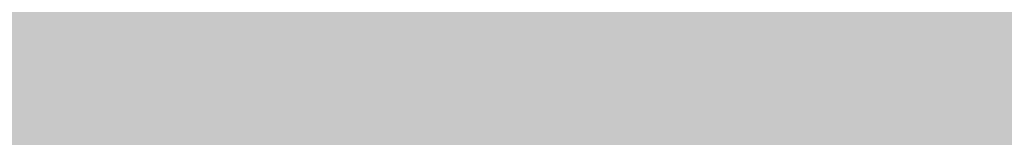
# Model space of a CAD drawing. Units: millimetres. Extents: x 0 to 2267, y 0 to 1823.
# Tile 199 of 256: x 1838.83 to 1841.442, y 1127.462 to 1127.775. Entities that reach past the tile are written whole.
import ezdxf

# ---------------------------------------------------------------- set-up
doc = ezdxf.new("R2010")
doc.units = ezdxf.units.MM
doc.header["$MEASUREMENT"] = 0
doc.layers.add('M-HATC', color=252, linetype='Continuous', lineweight=18)

msp = doc.modelspace()

# ---------------------------------------------------------------- hatches: boundary and pattern name
at = {"layer": 'M-HATC'}
h = msp.add_hatch(color=256, dxfattribs=at)
h.dxf.hatch_style = 1
h.paths.add_polyline_path([(2055.771, 1603.062), (1381.0868, 1603.062), (1381.0868, 1598.062), (2055.771, 1598.062)])
h.paths.add_polyline_path([(2055.771, 1598.062), (1381.0868, 1598.062), (1381.0868, 1593.062), (2055.771, 1593.062)])
h.paths.add_polyline_path([(2051.3074, 1536.7609), (1385.5504, 1536.7609), (1385.5504, 1526.7609), (1387.5504, 1526.7609), (1388.5366, 1525.0528), (1385.3319, 1521.2335), (1385.3319, 1521.2226), (2050.2542, 1522.7491), (2048.3212, 1525.0528), (2049.3074, 1526.7609), (2051.3074, 1526.7609)])
edge = h.paths.add_edge_path()
edge.add_arc((1847.5345, 1379.1492), 135, 222.603061, 222.890851, ccw=False)
edge.add_line((1748.1663, 1287.7656), (1683.0921, 1287.7656))
edge.add_arc((1583.7239, 1379.1492), 135, 317.109149, 317.396939, ccw=False)
edge.add_arc((1678.9686, 1290.6707), 5, 222.8909, 317.1091, ccw=False)
edge.add_arc((1774.2133, 1379.1492), 135, 222.603061, 222.890851, ccw=False)
edge.add_line((1674.8451, 1287.7656), (1609.7709, 1287.7656))
edge.add_arc((1510.4027, 1379.1492), 135, 317.109149, 317.396939, ccw=False)
edge.add_arc((1605.6474, 1290.6707), 5, 222.8909, 317.1091, ccw=False)
edge.add_arc((1700.8921, 1379.1492), 135, 222.603061, 222.890851, ccw=False)
edge.add_line((1601.5239, 1287.7656), (1536.4497, 1287.7656))
edge.add_arc((1437.0815, 1379.1492), 135, 317.109149, 317.396939, ccw=False)
edge.add_arc((1532.3262, 1290.6707), 5, 222.8909, 317.1091, ccw=False)
edge.add_arc((1627.5709, 1379.1492), 135, 222.603061, 222.890851, ccw=False)
edge.add_line((1528.2027, 1287.7656), (1505.9289, 1287.7656))
edge.add_spline(control_points=[(1505.9289, 1287.7656), (1504.2622, 1287.7656), (1504.2622, 1282.7656), (1505.9289, 1282.7656)], knot_values=[0, 0, 0, 0, 5, 5, 5, 5], degree=3, periodic=0)
edge.add_line((1505.9289, 1282.7656), (1930.9289, 1282.7656))
edge.add_spline(control_points=[(1930.9289, 1282.7656), (1932.5956, 1282.7656), (1932.5956, 1287.7656), (1930.9289, 1287.7656)], knot_values=[0, 0, 0, 0, 5, 5, 5, 5], degree=3, periodic=0)
edge.add_line((1930.9289, 1287.7656), (1903.0557, 1287.7656))
edge.add_arc((1803.6875, 1379.1492), 135, 317.109149, 317.396939, ccw=False)
edge.add_arc((1898.9322, 1290.6707), 5, 222.8909, 317.1091, ccw=False)
edge.add_arc((1994.1769, 1379.1492), 135, 222.603061, 222.890851, ccw=False)
edge.add_line((1894.8087, 1287.7656), (1829.7345, 1287.7656))
edge.add_arc((1730.3663, 1379.1492), 135, 317.109149, 317.396939, ccw=False)
edge.add_arc((1825.611, 1290.6707), 5, 222.8909, 317.1091, ccw=False)
edge.add_arc((1920.8557, 1379.1492), 135, 222.603061, 222.890851, ccw=False)
edge.add_line((1821.4875, 1287.7656), (1756.4133, 1287.7656))
edge.add_arc((1657.0451, 1379.1492), 135, 317.109149, 317.396939, ccw=False)
edge.add_arc((1752.2898, 1290.6707), 5, 222.8909, 317.1091, ccw=False)
edge = h.paths.add_edge_path()
edge.add_spline(control_points=[(1843.4289, 1227.2475), (1845.0956, 1227.2475), (1845.0956, 1232.2475), (1843.4289, 1232.2475)], knot_values=[0, 0, 0, 0, 5, 5, 5, 5], degree=3, periodic=0)
edge.add_line((1843.4289, 1232.2475), (1593.4289, 1232.2475))
edge.add_spline(control_points=[(1593.4289, 1232.2475), (1591.7622, 1232.2475), (1591.7622, 1227.2475), (1593.4289, 1227.2475)], knot_values=[0, 0, 0, 0, 5, 5, 5, 5], degree=3, periodic=0)
edge.add_line((1593.4289, 1227.2475), (1843.4289, 1227.2475))
h.paths.add_polyline_path([(1905.9289, 1127.4171), (1530.9289, 1127.4171, 0.414214), (1520.9289, 1117.4171), (1530.9289, 1117.4171), (1915.9289, 1117.4171, 0.414214)])
edge = h.paths.add_edge_path()
edge.add_arc((1397.0858, 1498.4078), 12.7299, 90.78215, 190.87871, ccw=False)
edge.add_line((1396.912, 1511.1365), (1428.0097, 1511.3488))
edge.add_line((1428.0097, 1511.3488), (1433.0097, 1511.3488))
edge.add_line((1433.0097, 1511.3488), (1434.439, 1511.3488))
edge.add_arc((1419.474, 1498.0804), 20, 41.561, 74.08211)
edge.add_line((1424.9592, 1517.3135), (1399.9351, 1517.2561))
edge.add_spline(control_points=[(1399.9307, 1517.2561), (1399.884, 1517.2131), (1399.8328, 1517.1689), (1399.7774, 1517.1236)], knot_values=[11.567499, 11.567499, 11.567499, 11.567499, 11.814249, 11.814249, 11.814249, 11.814249], degree=3, periodic=0)
edge.add_spline(control_points=[(1399.6328, 1517.0099), (1399.5831, 1516.9721), (1399.5307, 1516.9338), (1399.4759, 1516.8947)], knot_values=[11.167718, 11.167718, 11.167718, 11.167718, 11.365188, 11.365188, 11.365188, 11.365188], degree=3, periodic=0)
edge.add_spline(control_points=[(1399.3398, 1516.8001), (1399.1514, 1516.6719), (1398.9384, 1516.5377), (1398.704, 1516.3994)], knot_values=[10.376405, 10.376405, 10.376405, 10.376405, 11.00994, 11.00994, 11.00994, 11.00994], degree=3, periodic=0)
edge.add_spline(control_points=[(1398.6572, 1516.3719), (1398.5789, 1516.326), (1398.4983, 1516.2797), (1398.4155, 1516.2331)], knot_values=[10.125175, 10.125175, 10.125175, 10.125175, 10.334406, 10.334406, 10.334406, 10.334406], degree=3, periodic=0)
edge.add_spline(control_points=[(1398.2642, 1516.1487), (1398.196, 1516.1111), (1398.1263, 1516.0732), (1398.0555, 1516.0351)], knot_values=[9.832246, 9.832246, 9.832246, 9.832246, 9.999658, 9.999658, 9.999658, 9.999658], degree=3, periodic=0)
edge.add_spline(control_points=[(1397.9987, 1516.0048), (1397.7312, 1515.8621), (1397.446, 1515.7171), (1397.1466, 1515.5714)], knot_values=[9.161808, 9.161808, 9.161808, 9.161808, 9.787769, 9.787769, 9.787769, 9.787769], degree=3, periodic=0)
edge.add_spline(control_points=[(1397.1466, 1515.5714), (1396.8418, 1515.423), (1396.5222, 1515.274), (1396.1914, 1515.1262)], knot_values=[8.524455, 8.524455, 8.524455, 8.524455, 9.161808, 9.161808, 9.161808, 9.161808], degree=3, periodic=0)
edge.add_spline(control_points=[(1396.0777, 1515.0756), (1395.9854, 1515.0348), (1395.8922, 1514.994), (1395.7983, 1514.9534)], knot_values=[8.275193, 8.275193, 8.275193, 8.275193, 8.451726, 8.451726, 8.451726, 8.451726], degree=3, periodic=0)
edge.add_spline(control_points=[(1395.6018, 1514.8691), (1395.4997, 1514.8257), (1395.3968, 1514.7824), (1395.2932, 1514.7394)], knot_values=[7.962917, 7.962917, 7.962917, 7.962917, 8.152764, 8.152764, 8.152764, 8.152764], degree=3, periodic=0)
edge.add_spline(control_points=[(1395.2116, 1514.7057), (1394.8278, 1514.5475), (1394.4345, 1514.3929), (1394.0364, 1514.2442)], knot_values=[7.21254, 7.21254, 7.21254, 7.21254, 7.913148, 7.913148, 7.913148, 7.913148], degree=3, periodic=0)
edge.add_spline(control_points=[(1394.0364, 1514.2442), (1393.7076, 1514.1214), (1393.3754, 1514.0027), (1393.0427, 1513.8895)], knot_values=[6.633733, 6.633733, 6.633733, 6.633733, 7.21254, 7.21254, 7.21254, 7.21254], degree=3, periodic=0)
edge.add_spline(control_points=[(1392.8214, 1513.815), (1392.7198, 1513.7812), (1392.6181, 1513.7479), (1392.5166, 1513.7152)], knot_values=[6.328796, 6.328796, 6.328796, 6.328796, 6.505493, 6.505493, 6.505493, 6.505493], degree=3, periodic=0)
edge.add_spline(control_points=[(1392.5166, 1513.7152), (1392.3187, 1513.6515), (1392.1212, 1513.59), (1391.9244, 1513.531)], knot_values=[5.984605, 5.984605, 5.984605, 5.984605, 6.328796, 6.328796, 6.328796, 6.328796], degree=3, periodic=0)
edge.add_spline(control_points=[(1391.7915, 1513.4915), (1391.3122, 1513.3501), (1390.8384, 1513.2239), (1390.3784, 1513.1171)], knot_values=[5.066697, 5.066697, 5.066697, 5.066697, 5.907055, 5.907055, 5.907055, 5.907055], degree=3, periodic=0)
edge.add_spline(control_points=[(1390.3784, 1513.1171), (1390.1797, 1513.071), (1389.9836, 1513.0284), (1389.7907, 1512.9899)], knot_values=[4.70367, 4.70367, 4.70367, 4.70367, 5.066695, 5.066695, 5.066695, 5.066695], degree=3, periodic=0)
edge.add_spline(control_points=[(1389.422, 1512.9204), (1389.2459, 1512.8892), (1389.0729, 1512.8617), (1388.9036, 1512.8381)], knot_values=[4.130571, 4.130571, 4.130571, 4.130571, 4.469816, 4.469816, 4.469816, 4.469816], degree=3, periodic=0)
edge.add_spline(control_points=[(1388.9036, 1512.8381), (1388.591, 1512.7946), (1388.2911, 1512.7644), (1388.0071, 1512.7494)], knot_values=[3.504031, 3.504031, 3.504031, 3.504031, 4.130571, 4.130571, 4.130571, 4.130571], degree=3, periodic=0)
edge.add_spline(control_points=[(1387.9356, 1512.7459), (1387.8538, 1512.7423), (1387.7733, 1512.74), (1387.6944, 1512.739)], knot_values=[3.268866, 3.268866, 3.268866, 3.268866, 3.451164, 3.451164, 3.451164, 3.451164], degree=3, periodic=0)
edge.add_spline(control_points=[(1387.3351, 1512.7443), (1387.2076, 1512.7499), (1387.0847, 1512.7597), (1386.967, 1512.7739)], knot_values=[2.670686, 2.670686, 2.670686, 2.670686, 2.984, 2.984, 2.984, 2.984], degree=3, periodic=0)
edge.add_spline(control_points=[(1386.8327, 1512.7922), (1386.8209, 1512.7941), (1386.8092, 1512.7959), (1386.7975, 1512.7979)], knot_values=[2.516981, 2.516981, 2.516981, 2.516981, 2.549528, 2.549528, 2.549528, 2.549528], degree=3, periodic=0)
edge.add_spline(control_points=[(1386.4526, 1512.8735), (1386.4257, 1512.881), (1386.3993, 1512.889), (1386.3733, 1512.8972)], knot_values=[2.095869, 2.095869, 2.095869, 2.095869, 2.17941, 2.17941, 2.17941, 2.17941], degree=3, periodic=0)
edge.add_spline(control_points=[(1386.0691, 1513.0189), (1386.0634, 1513.0217), (1386.0577, 1513.0246), (1386.052, 1513.0275)], knot_values=[1.72453, 1.72453, 1.72453, 1.72453, 1.745933, 1.745933, 1.745933, 1.745933], degree=3, periodic=0)
edge.add_arc((1399.474, 1498.0804), 20, 131.82432, 180)
edge.add_arc((1630.3336, 1505.5484), 250.9708, 181.705176, 236.427975)
edge.add_arc((1605.3399, 1483.3044), 218.7822, 238.660829, 243.34961)
edge.add_arc((1647.0911, 1510.3592), 262.8986, 183.129836, 237.853442, ccw=False)
h.paths.add_polyline_path([(1406.5369, 1391.9644, 0.149382), (1491.5506, 1296.4418, -0.129517)], flags=17)
edge = h.paths.add_edge_path()
edge.add_arc((2037.3838, 1498.0804), 20, 0, 48.26587)
edge.add_spline(control_points=[(2050.6973, 1513.0052), (2050.6512, 1512.9847), (2050.6034, 1512.9655), (2050.5539, 1512.9477)], knot_values=[1.835652, 1.835652, 1.835652, 1.835652, 2.000781, 2.000781, 2.000781, 2.000781], degree=3, periodic=0)
edge.add_spline(control_points=[(2050.4616, 1512.9166), (2050.479, 1512.9221), (2050.4963, 1512.9277), (2050.5133, 1512.9335)], knot_values=[2.045477, 2.045477, 2.045477, 2.045477, 2.101389, 2.101389, 2.101389, 2.101389], degree=3, periodic=0)
edge.add_spline(control_points=[(2050.129, 1512.8342), (2050.1984, 1512.8473), (2050.2657, 1512.8623), (2050.3308, 1512.8792)], knot_values=[2.237629, 2.237629, 2.237629, 2.237629, 2.435841, 2.435841, 2.435841, 2.435841], degree=3, periodic=0)
edge.add_spline(control_points=[(2050.0946, 1512.8278), (2050.1061, 1512.8299), (2050.1176, 1512.832), (2050.129, 1512.8342)], knot_values=[2.435841, 2.435841, 2.435841, 2.435841, 2.468321, 2.468321, 2.468321, 2.468321], degree=3, periodic=0)
edge.add_spline(control_points=[(2049.7843, 1512.7851), (2049.8552, 1512.7922), (2049.9243, 1512.8008), (2049.9917, 1512.8109)], knot_values=[2.563852, 2.563852, 2.563852, 2.563852, 2.748541, 2.748541, 2.748541, 2.748541], degree=3, periodic=0)
edge.add_spline(control_points=[(2049.4052, 1512.7617), (2049.5364, 1512.7653), (2049.6629, 1512.773), (2049.7843, 1512.7851)], knot_values=[2.748541, 2.748541, 2.748541, 2.748541, 3.064882, 3.064882, 3.064882, 3.064882], degree=3, periodic=0)
edge.add_spline(control_points=[(2049.1698, 1512.7597), (2049.2336, 1512.7591), (2049.2965, 1512.7594), (2049.3584, 1512.7606)], knot_values=[3.102309, 3.102309, 3.102309, 3.102309, 3.2503, 3.2503, 3.2503, 3.2503], degree=3, periodic=0)
edge.add_spline(control_points=[(2048.8573, 1512.7691), (2048.9638, 1512.7638), (2049.068, 1512.7606), (2049.1698, 1512.7597)], knot_values=[3.2503, 3.2503, 3.2503, 3.2503, 3.486069, 3.486069, 3.486069, 3.486069], degree=3, periodic=0)
edge.add_spline(control_points=[(2048.6924, 1512.7789), (2048.3729, 1512.8009), (2048.0345, 1512.8411), (2047.6817, 1512.897)], knot_values=[3.606429, 3.606429, 3.606429, 3.606429, 4.2989, 4.2989, 4.2989, 4.2989], degree=3, periodic=0)
edge.add_spline(control_points=[(2047.6817, 1512.897), (2047.5458, 1512.9185), (2047.4077, 1512.9424), (2047.2678, 1512.9685)], knot_values=[4.2989, 4.2989, 4.2989, 4.2989, 4.565769, 4.565769, 4.565769, 4.565769], degree=3, periodic=0)
edge.add_spline(control_points=[(2047.2678, 1512.9685), (2047.1449, 1512.9914), (2047.0207, 1513.016), (2046.8951, 1513.0422)], knot_values=[4.565769, 4.565769, 4.565769, 4.565769, 4.799971, 4.799971, 4.799971, 4.799971], degree=3, periodic=0)
edge.add_spline(control_points=[(2046.8951, 1513.0422), (2046.5286, 1513.1188), (2046.1513, 1513.209), (2045.7676, 1513.3107)], knot_values=[4.799971, 4.799971, 4.799971, 4.799971, 5.483718, 5.483718, 5.483718, 5.483718], degree=3, periodic=0)
edge.add_spline(control_points=[(2045.7676, 1513.3107), (2045.3724, 1513.4154), (2044.9704, 1513.5322), (2044.5662, 1513.6588)], knot_values=[5.483718, 5.483718, 5.483718, 5.483718, 6.187866, 6.187866, 6.187866, 6.187866], degree=3, periodic=0)
edge.add_spline(control_points=[(2044.5662, 1513.6588), (2044.4149, 1513.7061), (2044.2633, 1513.7549), (2044.1116, 1513.8048)], knot_values=[6.187866, 6.187866, 6.187866, 6.187866, 6.451551, 6.451551, 6.451551, 6.451551], degree=3, periodic=0)
edge.add_spline(control_points=[(2044.1116, 1513.8048), (2043.9967, 1513.8427), (2043.8817, 1513.8813), (2043.7668, 1513.9205)], knot_values=[6.451551, 6.451551, 6.451551, 6.451551, 6.651434, 6.651434, 6.651434, 6.651434], degree=3, periodic=0)
edge.add_spline(control_points=[(2043.7668, 1513.9205), (2043.3716, 1514.0554), (2042.9774, 1514.1979), (2042.5886, 1514.3458)], knot_values=[6.651434, 6.651434, 6.651434, 6.651434, 7.338879, 7.338879, 7.338879, 7.338879], degree=3, periodic=0)
edge.add_spline(control_points=[(2042.5886, 1514.3458), (2042.1643, 1514.5071), (2041.7465, 1514.6749), (2041.3409, 1514.846)], knot_values=[7.338879, 7.338879, 7.338879, 7.338879, 8.089209, 8.089209, 8.089209, 8.089209], degree=3, periodic=0)
edge.add_spline(control_points=[(2041.3409, 1514.846), (2041.1028, 1514.9465), (2040.869, 1515.0481), (2040.6405, 1515.1502)], knot_values=[8.089209, 8.089209, 8.089209, 8.089209, 8.529587, 8.529587, 8.529587, 8.529587], degree=3, periodic=0)
edge.add_spline(control_points=[(2040.51, 1515.2089), (2040.0824, 1515.4022), (2039.6747, 1515.5971), (2039.295, 1515.7894)], knot_values=[8.613818, 8.613818, 8.613818, 8.613818, 9.44571, 9.44571, 9.44571, 9.44571], degree=3, periodic=0)
edge.add_spline(control_points=[(2039.295, 1515.7894), (2039.0618, 1515.9075), (2038.8391, 1516.0246), (2038.6288, 1516.1398)], knot_values=[9.44571, 9.44571, 9.44571, 9.44571, 9.956404, 9.956404, 9.956404, 9.956404], degree=3, periodic=0)
edge.add_spline(control_points=[(2038.6288, 1516.1398), (2038.5187, 1516.2001), (2038.4121, 1516.2598), (2038.309, 1516.3189)], knot_values=[9.956404, 9.956404, 9.956404, 9.956404, 10.223542, 10.223542, 10.223542, 10.223542], degree=3, periodic=0)
edge.add_spline(control_points=[(2038.309, 1516.3189), (2038.2138, 1516.3735), (2038.1216, 1516.4276), (2038.0328, 1516.481)], knot_values=[10.223542, 10.223542, 10.223542, 10.223542, 10.47051, 10.47051, 10.47051, 10.47051], degree=3, periodic=0)
edge.add_spline(control_points=[(2038.0328, 1516.481), (2037.7855, 1516.6296), (2037.5639, 1516.773), (2037.3722, 1516.909)], knot_values=[10.47051, 10.47051, 10.47051, 10.47051, 11.15767, 11.15767, 11.15767, 11.15767], degree=3, periodic=0)
edge.add_spline(control_points=[(2037.3722, 1516.909), (2037.2789, 1516.9752), (2037.1927, 1517.0396), (2037.1142, 1517.102)], knot_values=[11.15767, 11.15767, 11.15767, 11.15767, 11.49227, 11.49227, 11.49227, 11.49227], degree=3, periodic=0)
edge.add_spline(control_points=[(2036.8564, 1517.3259), (2036.9148, 1517.2692), (2036.9814, 1517.2103), (2037.0557, 1517.1492)], knot_values=[11.577341, 11.577341, 11.577341, 11.577341, 11.91035, 11.91035, 11.91035, 11.91035], degree=3, periodic=0)
edge.add_spline(control_points=[(2036.8074, 1517.3748), (2036.823, 1517.3587), (2036.8393, 1517.3424), (2036.8564, 1517.3259)], knot_values=[11.91035, 11.91035, 11.91035, 11.91035, 12.007402, 12.007402, 12.007402, 12.007402], degree=3, periodic=0)
edge.add_spline(control_points=[(2036.7017, 1517.494), (2036.7104, 1517.483), (2036.7196, 1517.4719), (2036.7291, 1517.4606)], knot_values=[12.184155, 12.184155, 12.184155, 12.184155, 12.255409, 12.255409, 12.255409, 12.255409], degree=3, periodic=0)
edge.add_spline(control_points=[(2036.6159, 1517.6205), (2036.62, 1517.613), (2036.6243, 1517.6055), (2036.6289, 1517.5979)], knot_values=[12.487913, 12.487913, 12.487913, 12.487913, 12.541035, 12.541035, 12.541035, 12.541035], degree=3, periodic=0)
edge.add_spline(control_points=[(2036.5635, 1517.786), (2036.5637, 1517.7794), (2036.5642, 1517.7726), (2036.565, 1517.7658)], knot_values=[12.911761, 12.911761, 12.911761, 12.911761, 12.968286, 12.968286, 12.968286, 12.968286], degree=3, periodic=0)
edge.add_spline(control_points=[(2036.6166, 1517.9304), (2036.6125, 1517.9259), (2036.6086, 1517.9212), (2036.6049, 1517.9165)], knot_values=[13.382527, 13.382527, 13.382527, 13.382527, 13.433791, 13.433791, 13.433791, 13.433791], degree=3, periodic=0)
edge.add_spline(control_points=[(2036.749, 1518.017), (2036.7361, 1518.0116), (2036.7239, 1518.006), (2036.7124, 1518.0002)], knot_values=[13.726299, 13.726299, 13.726299, 13.726299, 13.809928, 13.809928, 13.809928, 13.809928], degree=3, periodic=0)
edge.add_spline(control_points=[(2036.8604, 1518.0528), (2036.8386, 1518.0474), (2036.8181, 1518.0416), (2036.7988, 1518.0353)], knot_values=[13.910887, 13.910887, 13.910887, 13.910887, 14.02153, 14.02153, 14.02153, 14.02153], degree=3, periodic=0)
edge.add_line((2036.9639, 1518.0804), (2032.3838, 1518.0804))
edge.add_line((2032.3838, 1518.0804), (2027.3838, 1518.0804))
edge.add_line((2027.3838, 1518.0804), (2022.3838, 1518.0804))
edge.add_line((2022.3838, 1518.0804), (2017.3838, 1518.0804))
edge.add_arc((2017.3838, 1498.0804), 20, 90, 138.439)
edge.add_line((2002.4188, 1511.3488), (2003.8481, 1511.3488))
edge.add_line((2003.8481, 1511.3488), (2008.8481, 1511.3488))
edge.add_line((2008.8481, 1511.3488), (2039.772, 1511.1377))
edge.add_arc((2039.772, 1498.4078), 12.7299, -10.87871, 90, ccw=False)
edge.add_arc((1789.7668, 1510.3592), 262.8986, 302.146558, 356.870164, ccw=False)
edge.add_arc((1831.5179, 1483.3044), 218.7822, 296.65039, 301.339171)
edge.add_arc((1806.5242, 1505.5484), 250.9708, 303.572025, 358.294824)
h.paths.add_polyline_path([(2030.321, 1391.9644, -0.129517), (1945.3072, 1296.4418, 0.149382)], flags=17)
edge = h.paths.add_edge_path()
edge.add_spline(control_points=[(2037.2464, 1518.0821), (2037.2898, 1518.081), (2037.3355, 1518.0804), (2037.3838, 1518.0804)], knot_values=[0.000012, 0.000012, 0.000012, 0.000012, 0.144754, 0.144754, 0.144754, 0.144754], degree=3, periodic=0)
edge.add_line((2037.3357, 1518.0804), (2037.0096, 1518.0804))
edge.add_spline(control_points=[(2037.0096, 1518.0804), (2036.9822, 1518.0768), (2036.956, 1518.0727), (2036.9312, 1518.0681)], knot_values=[14.13465, 14.13465, 14.13465, 14.13465, 14.247197, 14.247197, 14.247197, 14.247197], degree=3, periodic=0)
edge.add_spline(control_points=[(2036.9312, 1518.0681), (2036.9276, 1518.0674), (2036.9241, 1518.0667), (2036.9205, 1518.0661)], knot_values=[14.118315, 14.118315, 14.118315, 14.118315, 14.13465, 14.13465, 14.13465, 14.13465], degree=3, periodic=0)
edge.add_spline(control_points=[(2036.9205, 1518.0661), (2036.9118, 1518.0644), (2036.9032, 1518.0626), (2036.8948, 1518.0608)], knot_values=[14.078086, 14.078086, 14.078086, 14.078086, 14.118315, 14.118315, 14.118315, 14.118315], degree=3, periodic=0)
edge.add_spline(control_points=[(2036.8948, 1518.0608), (2036.883, 1518.0583), (2036.8716, 1518.0556), (2036.8604, 1518.0528)], knot_values=[14.02153, 14.02153, 14.02153, 14.02153, 14.078086, 14.078086, 14.078086, 14.078086], degree=3, periodic=0)
edge.add_spline(control_points=[(2036.8604, 1518.0528), (2036.8386, 1518.0474), (2036.8181, 1518.0416), (2036.7988, 1518.0353)], knot_values=[13.910887, 13.910887, 13.910887, 13.910887, 14.02153, 14.02153, 14.02153, 14.02153], degree=3, periodic=0)
edge.add_spline(control_points=[(2036.7988, 1518.0353), (2036.7981, 1518.035), (2036.7974, 1518.0348), (2036.7967, 1518.0346)], knot_values=[13.906906, 13.906906, 13.906906, 13.906906, 13.910887, 13.910887, 13.910887, 13.910887], degree=3, periodic=0)
edge.add_spline(control_points=[(2036.7967, 1518.0346), (2036.7882, 1518.0318), (2036.7799, 1518.0289), (2036.7719, 1518.0259)], knot_values=[13.857826, 13.857826, 13.857826, 13.857826, 13.906906, 13.906906, 13.906906, 13.906906], degree=3, periodic=0)
edge.add_spline(control_points=[(2036.7719, 1518.0259), (2036.764, 1518.023), (2036.7564, 1518.02), (2036.749, 1518.017)], knot_values=[13.809928, 13.809928, 13.809928, 13.809928, 13.857826, 13.857826, 13.857826, 13.857826], degree=3, periodic=0)
edge.add_spline(control_points=[(2036.749, 1518.017), (2036.7361, 1518.0116), (2036.7239, 1518.006), (2036.7124, 1518.0002)], knot_values=[13.726299, 13.726299, 13.726299, 13.726299, 13.809928, 13.809928, 13.809928, 13.809928], degree=3, periodic=0)
edge.add_spline(control_points=[(2036.7124, 1518.0002), (2036.7121, 1518), (2036.7118, 1517.9999), (2036.7115, 1517.9997)], knot_values=[13.723993, 13.723993, 13.723993, 13.723993, 13.726299, 13.726299, 13.726299, 13.726299], degree=3, periodic=0)
edge.add_spline(control_points=[(2036.7115, 1517.9997), (2036.7063, 1517.9971), (2036.7013, 1517.9944), (2036.6965, 1517.9917)], knot_values=[13.686536, 13.686536, 13.686536, 13.686536, 13.723993, 13.723993, 13.723993, 13.723993], degree=3, periodic=0)
edge.add_spline(control_points=[(2036.6965, 1517.9917), (2036.6919, 1517.9891), (2036.6874, 1517.9865), (2036.6831, 1517.9839)], knot_values=[13.651251, 13.651251, 13.651251, 13.651251, 13.686536, 13.686536, 13.686536, 13.686536], degree=3, periodic=0)
edge.add_spline(control_points=[(2036.6831, 1517.9839), (2036.6764, 1517.9798), (2036.67, 1517.9757), (2036.6639, 1517.9714)], knot_values=[13.596804, 13.596804, 13.596804, 13.596804, 13.651251, 13.651251, 13.651251, 13.651251], degree=3, periodic=0)
edge.add_spline(control_points=[(2036.6639, 1517.9714), (2036.6636, 1517.9712), (2036.6633, 1517.9709), (2036.6629, 1517.9707)], knot_values=[13.593956, 13.593956, 13.593956, 13.593956, 13.596804, 13.596804, 13.596804, 13.596804], degree=3, periodic=0)
edge.add_spline(control_points=[(2036.6629, 1517.9707), (2036.6603, 1517.9689), (2036.6577, 1517.967), (2036.6552, 1517.9651)], knot_values=[13.570322, 13.570322, 13.570322, 13.570322, 13.593956, 13.593956, 13.593956, 13.593956], degree=3, periodic=0)
edge.add_spline(control_points=[(2036.6552, 1517.9651), (2036.6525, 1517.9631), (2036.6499, 1517.9611), (2036.6474, 1517.9591)], knot_values=[13.545477, 13.545477, 13.545477, 13.545477, 13.570322, 13.570322, 13.570322, 13.570322], degree=3, periodic=0)
edge.add_spline(control_points=[(2036.6474, 1517.9591), (2036.6472, 1517.9589), (2036.6471, 1517.9588), (2036.6469, 1517.9587)], knot_values=[13.543931, 13.543931, 13.543931, 13.543931, 13.545477, 13.545477, 13.545477, 13.545477], degree=3, periodic=0)
edge.add_spline(control_points=[(2036.6469, 1517.9587), (2036.6412, 1517.9541), (2036.6358, 1517.9494), (2036.6307, 1517.9447)], knot_values=[13.488237, 13.488237, 13.488237, 13.488237, 13.543931, 13.543931, 13.543931, 13.543931], degree=3, periodic=0)
edge.add_spline(control_points=[(2036.6307, 1517.9447), (2036.6282, 1517.9423), (2036.6257, 1517.9399), (2036.6233, 1517.9374)], knot_values=[13.460307, 13.460307, 13.460307, 13.460307, 13.488237, 13.488237, 13.488237, 13.488237], degree=3, periodic=0)
edge.add_spline(control_points=[(2036.6233, 1517.9374), (2036.6215, 1517.9356), (2036.6198, 1517.9338), (2036.6181, 1517.932)], knot_values=[13.439712, 13.439712, 13.439712, 13.439712, 13.460307, 13.460307, 13.460307, 13.460307], degree=3, periodic=0)
edge.add_spline(control_points=[(2036.6181, 1517.932), (2036.6176, 1517.9315), (2036.6171, 1517.9309), (2036.6166, 1517.9304)], knot_values=[13.433791, 13.433791, 13.433791, 13.433791, 13.439712, 13.439712, 13.439712, 13.439712], degree=3, periodic=0)
edge.add_spline(control_points=[(2036.6166, 1517.9304), (2036.6125, 1517.9259), (2036.6086, 1517.9212), (2036.6049, 1517.9165)], knot_values=[13.382527, 13.382527, 13.382527, 13.382527, 13.433791, 13.433791, 13.433791, 13.433791], degree=3, periodic=0)
edge.add_spline(control_points=[(2036.6049, 1517.9165), (2036.6026, 1517.9135), (2036.6004, 1517.9104), (2036.5982, 1517.9074)], knot_values=[13.350017, 13.350017, 13.350017, 13.350017, 13.382527, 13.382527, 13.382527, 13.382527], degree=3, periodic=0)
edge.add_spline(control_points=[(2036.5982, 1517.9074), (2036.5972, 1517.9059), (2036.5962, 1517.9043), (2036.5952, 1517.9028)], knot_values=[13.333922, 13.333922, 13.333922, 13.333922, 13.350017, 13.350017, 13.350017, 13.350017], degree=3, periodic=0)
edge.add_spline(control_points=[(2036.5952, 1517.9028), (2036.5945, 1517.9018), (2036.5939, 1517.9009), (2036.5933, 1517.8999)], knot_values=[13.323828, 13.323828, 13.323828, 13.323828, 13.333922, 13.333922, 13.333922, 13.333922], degree=3, periodic=0)
edge.add_spline(control_points=[(2036.5933, 1517.8999), (2036.5905, 1517.8955), (2036.5879, 1517.8909), (2036.5855, 1517.8864)], knot_values=[13.277545, 13.277545, 13.277545, 13.277545, 13.323828, 13.323828, 13.323828, 13.323828], degree=3, periodic=0)
edge.add_spline(control_points=[(2036.5855, 1517.8864), (2036.5836, 1517.8827), (2036.5817, 1517.8789), (2036.5801, 1517.8751)], knot_values=[13.240119, 13.240119, 13.240119, 13.240119, 13.277545, 13.277545, 13.277545, 13.277545], degree=3, periodic=0)
edge.add_spline(control_points=[(2036.5801, 1517.8751), (2036.5795, 1517.8739), (2036.579, 1517.8727), (2036.5785, 1517.8715)], knot_values=[13.228211, 13.228211, 13.228211, 13.228211, 13.240119, 13.240119, 13.240119, 13.240119], degree=3, periodic=0)
edge.add_spline(control_points=[(2036.5785, 1517.8715), (2036.578, 1517.8702), (2036.5774, 1517.869), (2036.5769, 1517.8677)], knot_values=[13.215717, 13.215717, 13.215717, 13.215717, 13.228211, 13.228211, 13.228211, 13.228211], degree=3, periodic=0)
edge.add_spline(control_points=[(2036.5769, 1517.8677), (2036.5755, 1517.864), (2036.5741, 1517.8603), (2036.5729, 1517.8565)], knot_values=[13.179847, 13.179847, 13.179847, 13.179847, 13.215717, 13.215717, 13.215717, 13.215717], degree=3, periodic=0)
edge.add_spline(control_points=[(2036.5729, 1517.8565), (2036.5713, 1517.8515), (2036.5699, 1517.8464), (2036.5687, 1517.8413)], knot_values=[13.132017, 13.132017, 13.132017, 13.132017, 13.179847, 13.179847, 13.179847, 13.179847], degree=3, periodic=0)
edge.add_spline(control_points=[(2036.5687, 1517.8413), (2036.5684, 1517.8402), (2036.5682, 1517.8392), (2036.568, 1517.8382)], knot_values=[13.122482, 13.122482, 13.122482, 13.122482, 13.132017, 13.132017, 13.132017, 13.132017], degree=3, periodic=0)
edge.add_spline(control_points=[(2036.568, 1517.8382), (2036.5676, 1517.8363), (2036.5672, 1517.8345), (2036.5669, 1517.8327)], knot_values=[13.105592, 13.105592, 13.105592, 13.105592, 13.122482, 13.122482, 13.122482, 13.122482], degree=3, periodic=0)
edge.add_spline(control_points=[(2036.5669, 1517.8327), (2036.5662, 1517.8292), (2036.5657, 1517.8257), (2036.5652, 1517.8222)], knot_values=[13.074063, 13.074063, 13.074063, 13.074063, 13.105592, 13.105592, 13.105592, 13.105592], degree=3, periodic=0)
edge.add_spline(control_points=[(2036.5652, 1517.8222), (2036.5652, 1517.8222), (2036.5652, 1517.8222), (2036.5652, 1517.8222)], knot_values=[13.074043, 13.074043, 13.074043, 13.074043, 13.074063, 13.074063, 13.074063, 13.074063], degree=3, periodic=0)
edge.add_spline(control_points=[(2036.5652, 1517.8222), (2036.5644, 1517.8164), (2036.5639, 1517.8106), (2036.5636, 1517.8046)], knot_values=[13.021884, 13.021884, 13.021884, 13.021884, 13.074043, 13.074043, 13.074043, 13.074043], degree=3, periodic=0)
edge.add_spline(control_points=[(2036.5636, 1517.8046), (2036.5636, 1517.804), (2036.5636, 1517.8034), (2036.5635, 1517.8028)], knot_values=[13.01674, 13.01674, 13.01674, 13.01674, 13.021884, 13.021884, 13.021884, 13.021884], degree=3, periodic=0)
edge.add_spline(control_points=[(2036.5635, 1517.8028), (2036.5634, 1517.8005), (2036.5634, 1517.7982), (2036.5634, 1517.7958)], knot_values=[12.996438, 12.996438, 12.996438, 12.996438, 13.01674, 13.01674, 13.01674, 13.01674], degree=3, periodic=0)
edge.add_spline(control_points=[(2036.5634, 1517.7958), (2036.5633, 1517.7926), (2036.5634, 1517.7893), (2036.5635, 1517.786)], knot_values=[12.968286, 12.968286, 12.968286, 12.968286, 12.996438, 12.996438, 12.996438, 12.996438], degree=3, periodic=0)
edge.add_spline(control_points=[(2036.5635, 1517.786), (2036.5637, 1517.7794), (2036.5642, 1517.7726), (2036.565, 1517.7658)], knot_values=[12.911761, 12.911761, 12.911761, 12.911761, 12.968286, 12.968286, 12.968286, 12.968286], degree=3, periodic=0)
edge.add_spline(control_points=[(2036.565, 1517.7658), (2036.565, 1517.7657), (2036.565, 1517.7656), (2036.565, 1517.7656)], knot_values=[12.911017, 12.911017, 12.911017, 12.911017, 12.911761, 12.911761, 12.911761, 12.911761], degree=3, periodic=0)
edge.add_spline(control_points=[(2036.565, 1517.7656), (2036.5654, 1517.7625), (2036.5658, 1517.7593), (2036.5663, 1517.7562)], knot_values=[12.88528, 12.88528, 12.88528, 12.88528, 12.911017, 12.911017, 12.911017, 12.911017], degree=3, periodic=0)
edge.add_spline(control_points=[(2036.5663, 1517.7562), (2036.5667, 1517.7534), (2036.5672, 1517.7506), (2036.5677, 1517.7478)], knot_values=[12.862519, 12.862519, 12.862519, 12.862519, 12.88528, 12.88528, 12.88528, 12.88528], degree=3, periodic=0)
edge.add_spline(control_points=[(2036.5677, 1517.7478), (2036.5678, 1517.7474), (2036.5679, 1517.7469), (2036.568, 1517.7465)], knot_values=[12.858885, 12.858885, 12.858885, 12.858885, 12.862519, 12.862519, 12.862519, 12.862519], degree=3, periodic=0)
edge.add_spline(control_points=[(2036.568, 1517.7465), (2036.5692, 1517.7399), (2036.5707, 1517.7332), (2036.5724, 1517.7264)], knot_values=[12.8053, 12.8053, 12.8053, 12.8053, 12.858885, 12.858885, 12.858885, 12.858885], degree=3, periodic=0)
edge.add_spline(control_points=[(2036.5724, 1517.7264), (2036.5734, 1517.7226), (2036.5745, 1517.7187), (2036.5756, 1517.7149)], knot_values=[12.775176, 12.775176, 12.775176, 12.775176, 12.8053, 12.8053, 12.8053, 12.8053], degree=3, periodic=0)
edge.add_spline(control_points=[(2036.5756, 1517.7149), (2036.5763, 1517.7125), (2036.577, 1517.7102), (2036.5778, 1517.7078)], knot_values=[12.756759, 12.756759, 12.756759, 12.756759, 12.775176, 12.775176, 12.775176, 12.775176], degree=3, periodic=0)
edge.add_spline(control_points=[(2036.5778, 1517.7078), (2036.5781, 1517.7067), (2036.5784, 1517.7057), (2036.5787, 1517.7047)], knot_values=[12.748742, 12.748742, 12.748742, 12.748742, 12.756759, 12.756759, 12.756759, 12.756759], degree=3, periodic=0)
edge.add_spline(control_points=[(2036.5787, 1517.7047), (2036.5808, 1517.6983), (2036.5831, 1517.6919), (2036.5856, 1517.6854)], knot_values=[12.69959, 12.69959, 12.69959, 12.69959, 12.748742, 12.748742, 12.748742, 12.748742], degree=3, periodic=0)
edge.add_spline(control_points=[(2036.5856, 1517.6854), (2036.5876, 1517.68), (2036.5898, 1517.6746), (2036.5921, 1517.6692)], knot_values=[12.659038, 12.659038, 12.659038, 12.659038, 12.69959, 12.69959, 12.69959, 12.69959], degree=3, periodic=0)
edge.add_spline(control_points=[(2036.5921, 1517.6692), (2036.594, 1517.6648), (2036.5959, 1517.6605), (2036.5979, 1517.6561)], knot_values=[12.626806, 12.626806, 12.626806, 12.626806, 12.659038, 12.659038, 12.659038, 12.659038], degree=3, periodic=0)
edge.add_spline(control_points=[(2036.5979, 1517.6561), (2036.5984, 1517.6551), (2036.5989, 1517.6541), (2036.5993, 1517.6531)], knot_values=[12.619394, 12.619394, 12.619394, 12.619394, 12.626806, 12.626806, 12.626806, 12.626806], degree=3, periodic=0)
edge.add_spline(control_points=[(2036.5993, 1517.6531), (2036.6043, 1517.6424), (2036.6099, 1517.6315), (2036.6159, 1517.6205)], knot_values=[12.541039, 12.541039, 12.541039, 12.541039, 12.619394, 12.619394, 12.619394, 12.619394], degree=3, periodic=0)
edge.add_spline(control_points=[(2036.6159, 1517.6205), (2036.6159, 1517.6205), (2036.6159, 1517.6205), (2036.6159, 1517.6205)], knot_values=[12.541035, 12.541035, 12.541035, 12.541035, 12.541039, 12.541039, 12.541039, 12.541039], degree=3, periodic=0)
edge.add_spline(control_points=[(2036.6159, 1517.6205), (2036.62, 1517.613), (2036.6243, 1517.6055), (2036.6289, 1517.5979)], knot_values=[12.487913, 12.487913, 12.487913, 12.487913, 12.541035, 12.541035, 12.541035, 12.541035], degree=3, periodic=0)
edge.add_spline(control_points=[(2036.6289, 1517.5979), (2036.6326, 1517.5916), (2036.6365, 1517.5853), (2036.6406, 1517.5789)], knot_values=[12.443982, 12.443982, 12.443982, 12.443982, 12.487913, 12.487913, 12.487913, 12.487913], degree=3, periodic=0)
edge.add_spline(control_points=[(2036.6406, 1517.5789), (2036.6414, 1517.5776), (2036.6423, 1517.5763), (2036.6431, 1517.5749)], knot_values=[12.434996, 12.434996, 12.434996, 12.434996, 12.443982, 12.443982, 12.443982, 12.443982], degree=3, periodic=0)
edge.add_spline(control_points=[(2036.6431, 1517.5749), (2036.6531, 1517.5596), (2036.6639, 1517.5439), (2036.6756, 1517.528)], knot_values=[12.329647, 12.329647, 12.329647, 12.329647, 12.434996, 12.434996, 12.434996, 12.434996], degree=3, periodic=0)
edge.add_spline(control_points=[(2036.6756, 1517.528), (2036.6839, 1517.5168), (2036.6925, 1517.5055), (2036.7017, 1517.494)], knot_values=[12.255409, 12.255409, 12.255409, 12.255409, 12.329647, 12.329647, 12.329647, 12.329647], degree=3, periodic=0)
edge.add_spline(control_points=[(2036.7017, 1517.494), (2036.7104, 1517.483), (2036.7196, 1517.4719), (2036.7291, 1517.4606)], knot_values=[12.184155, 12.184155, 12.184155, 12.184155, 12.255409, 12.255409, 12.255409, 12.255409], degree=3, periodic=0)
edge.add_spline(control_points=[(2036.7291, 1517.4606), (2036.7436, 1517.4435), (2036.759, 1517.4262), (2036.7753, 1517.4085)], knot_values=[12.075961, 12.075961, 12.075961, 12.075961, 12.184155, 12.184155, 12.184155, 12.184155], degree=3, periodic=0)
edge.add_spline(control_points=[(2036.7753, 1517.4085), (2036.7763, 1517.4075), (2036.7773, 1517.4064), (2036.7783, 1517.4054)], knot_values=[12.069502, 12.069502, 12.069502, 12.069502, 12.075961, 12.075961, 12.075961, 12.075961], degree=3, periodic=0)
edge.add_spline(control_points=[(2036.7783, 1517.4054), (2036.7877, 1517.3953), (2036.7974, 1517.385), (2036.8074, 1517.3748)], knot_values=[12.007402, 12.007402, 12.007402, 12.007402, 12.069502, 12.069502, 12.069502, 12.069502], degree=3, periodic=0)
edge.add_spline(control_points=[(2036.8074, 1517.3748), (2036.823, 1517.3587), (2036.8393, 1517.3424), (2036.8564, 1517.3259)], knot_values=[11.91035, 11.91035, 11.91035, 11.91035, 12.007402, 12.007402, 12.007402, 12.007402], degree=3, periodic=0)
edge.add_spline(control_points=[(2036.8564, 1517.3259), (2036.9148, 1517.2692), (2036.9814, 1517.2103), (2037.0557, 1517.1492)], knot_values=[11.577341, 11.577341, 11.577341, 11.577341, 11.91035, 11.91035, 11.91035, 11.91035], degree=3, periodic=0)
edge.add_spline(control_points=[(2037.0557, 1517.1492), (2037.0747, 1517.1336), (2037.0942, 1517.1179), (2037.1142, 1517.102)], knot_values=[11.49227, 11.49227, 11.49227, 11.49227, 11.577341, 11.577341, 11.577341, 11.577341], degree=3, periodic=0)
edge.add_spline(control_points=[(2037.1142, 1517.102), (2037.1927, 1517.0396), (2037.2789, 1516.9752), (2037.3722, 1516.909)], knot_values=[11.15767, 11.15767, 11.15767, 11.15767, 11.49227, 11.49227, 11.49227, 11.49227], degree=3, periodic=0)
edge.add_spline(control_points=[(2037.3722, 1516.909), (2037.5639, 1516.773), (2037.7855, 1516.6296), (2038.0328, 1516.481)], knot_values=[10.47051, 10.47051, 10.47051, 10.47051, 11.15767, 11.15767, 11.15767, 11.15767], degree=3, periodic=0)
edge.add_spline(control_points=[(2038.0328, 1516.481), (2038.1216, 1516.4276), (2038.2138, 1516.3735), (2038.309, 1516.3189)], knot_values=[10.223542, 10.223542, 10.223542, 10.223542, 10.47051, 10.47051, 10.47051, 10.47051], degree=3, periodic=0)
edge.add_spline(control_points=[(2038.309, 1516.3189), (2038.4121, 1516.2598), (2038.5187, 1516.2001), (2038.6288, 1516.1398)], knot_values=[9.956404, 9.956404, 9.956404, 9.956404, 10.223542, 10.223542, 10.223542, 10.223542], degree=3, periodic=0)
edge.add_spline(control_points=[(2038.6288, 1516.1398), (2038.8391, 1516.0246), (2039.0618, 1515.9075), (2039.295, 1515.7894)], knot_values=[9.44571, 9.44571, 9.44571, 9.44571, 9.956404, 9.956404, 9.956404, 9.956404], degree=3, periodic=0)
edge.add_spline(control_points=[(2039.295, 1515.7894), (2039.6747, 1515.5971), (2040.0824, 1515.4022), (2040.51, 1515.2089)], knot_values=[8.613818, 8.613818, 8.613818, 8.613818, 9.44571, 9.44571, 9.44571, 9.44571], degree=3, periodic=0)
edge.add_spline(control_points=[(2040.51, 1515.2089), (2040.5533, 1515.1893), (2040.5968, 1515.1697), (2040.6405, 1515.1502)], knot_values=[8.529587, 8.529587, 8.529587, 8.529587, 8.613818, 8.613818, 8.613818, 8.613818], degree=3, periodic=0)
edge.add_spline(control_points=[(2040.6405, 1515.1502), (2040.869, 1515.0481), (2041.1028, 1514.9465), (2041.3409, 1514.846)], knot_values=[8.089209, 8.089209, 8.089209, 8.089209, 8.529587, 8.529587, 8.529587, 8.529587], degree=3, periodic=0)
edge.add_spline(control_points=[(2041.3409, 1514.846), (2041.7465, 1514.6749), (2042.1643, 1514.5071), (2042.5886, 1514.3458)], knot_values=[7.338879, 7.338879, 7.338879, 7.338879, 8.089209, 8.089209, 8.089209, 8.089209], degree=3, periodic=0)
edge.add_spline(control_points=[(2042.5886, 1514.3458), (2042.9774, 1514.1979), (2043.3716, 1514.0554), (2043.7668, 1513.9205)], knot_values=[6.651434, 6.651434, 6.651434, 6.651434, 7.338879, 7.338879, 7.338879, 7.338879], degree=3, periodic=0)
edge.add_spline(control_points=[(2043.7668, 1513.9205), (2043.8817, 1513.8813), (2043.9967, 1513.8427), (2044.1116, 1513.8048)], knot_values=[6.451551, 6.451551, 6.451551, 6.451551, 6.651434, 6.651434, 6.651434, 6.651434], degree=3, periodic=0)
edge.add_spline(control_points=[(2044.1116, 1513.8048), (2044.2633, 1513.7549), (2044.4149, 1513.7061), (2044.5662, 1513.6588)], knot_values=[6.187866, 6.187866, 6.187866, 6.187866, 6.451551, 6.451551, 6.451551, 6.451551], degree=3, periodic=0)
edge.add_spline(control_points=[(2044.5662, 1513.6588), (2044.9704, 1513.5322), (2045.3724, 1513.4154), (2045.7676, 1513.3107)], knot_values=[5.483718, 5.483718, 5.483718, 5.483718, 6.187866, 6.187866, 6.187866, 6.187866], degree=3, periodic=0)
edge.add_spline(control_points=[(2045.7676, 1513.3107), (2046.1513, 1513.209), (2046.5286, 1513.1188), (2046.8951, 1513.0422)], knot_values=[4.799971, 4.799971, 4.799971, 4.799971, 5.483718, 5.483718, 5.483718, 5.483718], degree=3, periodic=0)
edge.add_spline(control_points=[(2046.8951, 1513.0422), (2047.0207, 1513.016), (2047.1449, 1512.9914), (2047.2678, 1512.9685)], knot_values=[4.565769, 4.565769, 4.565769, 4.565769, 4.799971, 4.799971, 4.799971, 4.799971], degree=3, periodic=0)
edge.add_spline(control_points=[(2047.2678, 1512.9685), (2047.4077, 1512.9424), (2047.5458, 1512.9185), (2047.6817, 1512.897)], knot_values=[4.2989, 4.2989, 4.2989, 4.2989, 4.565769, 4.565769, 4.565769, 4.565769], degree=3, periodic=0)
edge.add_spline(control_points=[(2047.6817, 1512.897), (2048.0345, 1512.8411), (2048.3729, 1512.8009), (2048.6924, 1512.7789)], knot_values=[3.606429, 3.606429, 3.606429, 3.606429, 4.2989, 4.2989, 4.2989, 4.2989], degree=3, periodic=0)
edge.add_spline(control_points=[(2048.6924, 1512.7789), (2048.7479, 1512.7751), (2048.8029, 1512.7718), (2048.8573, 1512.7691)], knot_values=[3.486069, 3.486069, 3.486069, 3.486069, 3.606429, 3.606429, 3.606429, 3.606429], degree=3, periodic=0)
edge.add_spline(control_points=[(2048.8573, 1512.7691), (2048.9638, 1512.7638), (2049.068, 1512.7606), (2049.1698, 1512.7597)], knot_values=[3.2503, 3.2503, 3.2503, 3.2503, 3.486069, 3.486069, 3.486069, 3.486069], degree=3, periodic=0)
edge.add_spline(control_points=[(2049.1698, 1512.7597), (2049.2336, 1512.7591), (2049.2965, 1512.7594), (2049.3584, 1512.7606)], knot_values=[3.102309, 3.102309, 3.102309, 3.102309, 3.2503, 3.2503, 3.2503, 3.2503], degree=3, periodic=0)
edge.add_spline(control_points=[(2049.3584, 1512.7606), (2049.3741, 1512.7609), (2049.3897, 1512.7613), (2049.4052, 1512.7617)], knot_values=[3.064882, 3.064882, 3.064882, 3.064882, 3.102309, 3.102309, 3.102309, 3.102309], degree=3, periodic=0)
edge.add_spline(control_points=[(2049.4052, 1512.7617), (2049.5364, 1512.7653), (2049.6629, 1512.773), (2049.7843, 1512.7851)], knot_values=[2.748541, 2.748541, 2.748541, 2.748541, 3.064882, 3.064882, 3.064882, 3.064882], degree=3, periodic=0)
edge.add_spline(control_points=[(2049.7843, 1512.7851), (2049.8552, 1512.7922), (2049.9243, 1512.8008), (2049.9917, 1512.8109)], knot_values=[2.563852, 2.563852, 2.563852, 2.563852, 2.748541, 2.748541, 2.748541, 2.748541], degree=3, periodic=0)
edge.add_spline(control_points=[(2049.9917, 1512.8109), (2050.0265, 1512.8161), (2050.0608, 1512.8218), (2050.0946, 1512.8278)], knot_values=[2.468321, 2.468321, 2.468321, 2.468321, 2.563852, 2.563852, 2.563852, 2.563852], degree=3, periodic=0)
edge.add_spline(control_points=[(2050.0946, 1512.8278), (2050.1061, 1512.8299), (2050.1176, 1512.832), (2050.129, 1512.8342)], knot_values=[2.435841, 2.435841, 2.435841, 2.435841, 2.468321, 2.468321, 2.468321, 2.468321], degree=3, periodic=0)
edge.add_spline(control_points=[(2050.129, 1512.8342), (2050.1984, 1512.8473), (2050.2657, 1512.8623), (2050.3308, 1512.8792)], knot_values=[2.237629, 2.237629, 2.237629, 2.237629, 2.435841, 2.435841, 2.435841, 2.435841], degree=3, periodic=0)
edge.add_spline(control_points=[(2050.3308, 1512.8792), (2050.3754, 1512.8908), (2050.4191, 1512.9032), (2050.4616, 1512.9166)], knot_values=[2.101389, 2.101389, 2.101389, 2.101389, 2.237629, 2.237629, 2.237629, 2.237629], degree=3, periodic=0)
edge.add_spline(control_points=[(2050.4616, 1512.9166), (2050.479, 1512.9221), (2050.4963, 1512.9277), (2050.5133, 1512.9335)], knot_values=[2.045477, 2.045477, 2.045477, 2.045477, 2.101389, 2.101389, 2.101389, 2.101389], degree=3, periodic=0)
edge.add_spline(control_points=[(2050.5133, 1512.9335), (2050.527, 1512.9382), (2050.5405, 1512.9429), (2050.5539, 1512.9477)], knot_values=[2.000781, 2.000781, 2.000781, 2.000781, 2.045477, 2.045477, 2.045477, 2.045477], degree=3, periodic=0)
edge.add_spline(control_points=[(2050.5539, 1512.9477), (2050.6034, 1512.9655), (2050.6512, 1512.9847), (2050.6973, 1513.0052)], knot_values=[1.835652, 1.835652, 1.835652, 1.835652, 2.000781, 2.000781, 2.000781, 2.000781], degree=3, periodic=0)
edge.add_arc((2037.3838, 1498.0804), 20, 48.26587, 90.12993)
edge = h.paths.add_edge_path(flags=16)
edge.add_spline(control_points=[(1386.1389, 1512.9859), (1388.92, 1511.7395), (1398.0387, 1515.5187), (1399.9307, 1517.2561)], knot_values=[1.831046, 1.831046, 1.831046, 1.831046, 11.814249, 11.814249, 11.814249, 11.814249], degree=3, periodic=0)
edge.add_line((1399.9307, 1517.2561), (1393.7435, 1517.2419))
edge.add_arc((1399.474, 1498.0804), 20, 106.6501, 131.8173)
h = msp.add_hatch(color=256, dxfattribs=at)
h.dxf.hatch_style = 1
h.paths.add_polyline_path([(2042.8886, 1580.1796), (2055.771, 1593.062), (1381.0868, 1593.062), (1393.9692, 1580.1796), (1374.086, 1560.2964), (2062.7718, 1560.2964)])
h.paths.add_polyline_path([(1843.4289, 1201.3297), (1843.4289, 1227.2475), (1593.4289, 1227.2475), (1593.4289, 1201.3297, -0.228274), (1574.5989, 1162.2346), (1530.9289, 1127.4171), (1905.9289, 1127.4171), (1862.2589, 1162.2346, -0.228274)])

doc.saveas('drawing.dxf')
